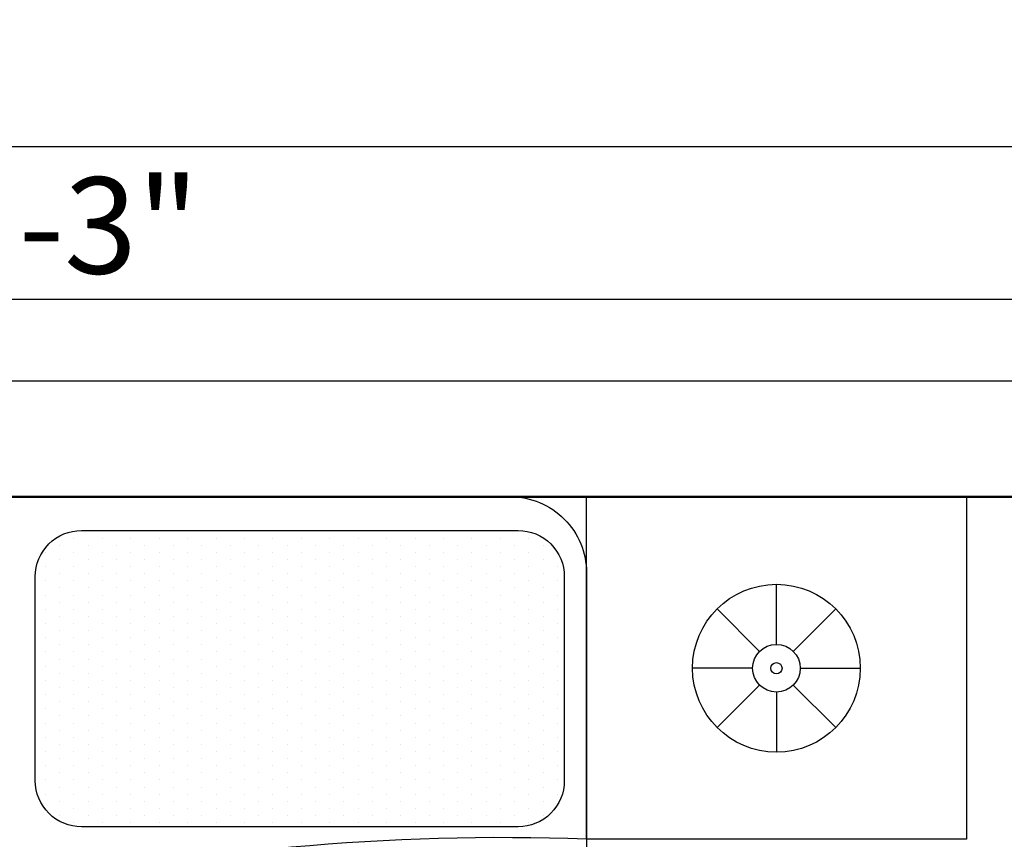
# Model space of a CAD drawing. Units: inches. Extents: x 3064 to 19385, y 846 to 15425.
# Tile 33 of 108: x 5003 to 5054, y 1368 to 1411. Entities that reach past the tile are written whole.
import ezdxf

# ---------------------------------------------------------------- set-up
doc = ezdxf.new("R2010")
doc.units = ezdxf.units.IN
for name, color, linetype, lineweight in [('A-ANNO-DIMS', 2, 'Continuous', 18), ('A-FLOR-FIXT', 9, 'Continuous', 18), ('A-WALL', 7, 'Continuous', 50), ('C-PROP', 6, 'Continuous', 25)]:
    doc.layers.add(name, color=color, linetype=linetype, lineweight=lineweight)
doc.layers.add('BLOCK', color=6, linetype='Continuous')
doc.styles.get("Standard").update_dxf_attribs({"font": 'arial.ttf'})
doc.dimstyles.new('ISO-25', dxfattribs={"dimtxt": 9, "dimasz": 2.5, "dimexe": 1.25, "dimexo": 0.625, "dimtad": 1, "dimdec": 1, "dimlunit": 3, "dimtxsty": 'Standard', "dimcen": 2.5, "dimadec": 0, "dimazin": 0, "dimtfac": 1, "dimtdec": 1, "dimtmove": 0, "dimatfit": 3, "dimfxl": 1, "dimarcsym": 0})

# ---------------------------------------------------------------- blocks, each defined once
blk = doc.blocks.new('*X7')
at = {"color": 0}
for p, q in [((273.75, 456.9375), (273.75, 456.9375)), ((273.9375, 457.03125), (273.9375, 457.03125)), ((274.125, 456.9375), (274.125, 456.9375)), ((274.3125, 457.03125), (274.3125, 457.03125)), ((274.5, 456.9375), (274.5, 456.9375)), ((274.6875, 457.03125), (274.6875, 457.03125)), ((274.875, 456.9375), (274.875, 456.9375)), ((275.0625, 457.03125), (275.0625, 457.03125)), ((275.25, 456.9375), (275.25, 456.9375)), ((275.4375, 457.03125), (275.4375, 457.03125)), ((275.625, 456.9375), (275.625, 456.9375)), ((275.8125, 457.03125), (275.8125, 457.03125)), ((276, 456.9375), (276, 456.9375)), ((276.1875, 457.03125), (276.1875, 457.03125)), ((276.375, 456.9375), (276.375, 456.9375)), ((276.5625, 457.03125), (276.5625, 457.03125)), ((276.75, 456.9375), (276.75, 456.9375)), ((276.9375, 457.03125), (276.9375, 457.03125)), ((277.125, 456.9375), (277.125, 456.9375)), ((277.3125, 457.03125), (277.3125, 457.03125)), ((277.5, 456.9375), (277.5, 456.9375)), ((277.6875, 457.03125), (277.6875, 457.03125)), ((277.875, 456.9375), (277.875, 456.9375)), ((278.0625, 457.03125), (278.0625, 457.03125)), ((278.25, 456.9375), (278.25, 456.9375)), ((278.4375, 457.03125), (278.4375, 457.03125)), ((278.625, 456.9375), (278.625, 456.9375)), ((278.8125, 457.03125), (278.8125, 457.03125)), ((279, 456.9375), (279, 456.9375)), ((279.1875, 457.03125), (279.1875, 457.03125)), ((279.375, 456.9375), (279.375, 456.9375)), ((279.5625, 457.03125), (279.5625, 457.03125)), ((279.75, 456.9375), (279.75, 456.9375)), ((273.5625, 456.84375), (273.5625, 456.84375)), ((273.9375, 456.84375), (273.9375, 456.84375)), ((274.3125, 456.84375), (274.3125, 456.84375)), ((274.6875, 456.84375), (274.6875, 456.84375)), ((275.0625, 456.84375), (275.0625, 456.84375)), ((275.4375, 456.84375), (275.4375, 456.84375)), ((275.8125, 456.84375), (275.8125, 456.84375)), ((276.1875, 456.84375), (276.1875, 456.84375)), ((276.5625, 456.84375), (276.5625, 456.84375)), ((276.9375, 456.84375), (276.9375, 456.84375)), ((277.3125, 456.84375), (277.3125, 456.84375)), ((277.6875, 456.84375), (277.6875, 456.84375)), ((278.0625, 456.84375), (278.0625, 456.84375)), ((278.4375, 456.84375), (278.4375, 456.84375)), ((278.8125, 456.84375), (278.8125, 456.84375)), ((279.1875, 456.84375), (279.1875, 456.84375)), ((279.5625, 456.84375), (279.5625, 456.84375)), ((279.9375, 456.84375), (279.9375, 456.84375)), ((273.375, 456.75), (273.375, 456.75)), ((273.5625, 456.65625), (273.5625, 456.65625)), ((273.75, 456.75), (273.75, 456.75)), ((273.9375, 456.65625), (273.9375, 456.65625)), ((274.125, 456.75), (274.125, 456.75)), ((274.3125, 456.65625), (274.3125, 456.65625)), ((274.5, 456.75), (274.5, 456.75)), ((274.6875, 456.65625), (274.6875, 456.65625)), ((274.875, 456.75), (274.875, 456.75)), ((275.0625, 456.65625), (275.0625, 456.65625)), ((275.25, 456.75), (275.25, 456.75)), ((275.4375, 456.65625), (275.4375, 456.65625)), ((275.625, 456.75), (275.625, 456.75)), ((275.8125, 456.65625), (275.8125, 456.65625)), ((276, 456.75), (276, 456.75)), ((276.1875, 456.65625), (276.1875, 456.65625)), ((276.375, 456.75), (276.375, 456.75)), ((276.5625, 456.65625), (276.5625, 456.65625)), ((276.75, 456.75), (276.75, 456.75)), ((276.9375, 456.65625), (276.9375, 456.65625)), ((277.125, 456.75), (277.125, 456.75)), ((277.3125, 456.65625), (277.3125, 456.65625)), ((277.5, 456.75), (277.5, 456.75)), ((277.6875, 456.65625), (277.6875, 456.65625)), ((277.875, 456.75), (277.875, 456.75)), ((278.0625, 456.65625), (278.0625, 456.65625)), ((278.25, 456.75), (278.25, 456.75)), ((278.4375, 456.65625), (278.4375, 456.65625)), ((278.625, 456.75), (278.625, 456.75)), ((278.8125, 456.65625), (278.8125, 456.65625)), ((279, 456.75), (279, 456.75)), ((279.1875, 456.65625), (279.1875, 456.65625)), ((279.375, 456.75), (279.375, 456.75)), ((279.5625, 456.65625), (279.5625, 456.65625)), ((279.75, 456.75), (279.75, 456.75)), ((279.9375, 456.65625), (279.9375, 456.65625)), ((280.125, 456.75), (280.125, 456.75)), ((273.375, 456.5625), (273.375, 456.5625)), ((273.75, 456.5625), (273.75, 456.5625)), ((274.125, 456.5625), (274.125, 456.5625)), ((274.5, 456.5625), (274.5, 456.5625)), ((274.875, 456.5625), (274.875, 456.5625)), ((275.25, 456.5625), (275.25, 456.5625)), ((275.625, 456.5625), (275.625, 456.5625)), ((276, 456.5625), (276, 456.5625)), ((276.375, 456.5625), (276.375, 456.5625)), ((276.75, 456.5625), (276.75, 456.5625)), ((277.125, 456.5625), (277.125, 456.5625)), ((277.5, 456.5625), (277.5, 456.5625)), ((277.875, 456.5625), (277.875, 456.5625)), ((278.25, 456.5625), (278.25, 456.5625)), ((278.625, 456.5625), (278.625, 456.5625)), ((279, 456.5625), (279, 456.5625)), ((279.375, 456.5625), (279.375, 456.5625)), ((279.75, 456.5625), (279.75, 456.5625)), ((280.125, 456.5625), (280.125, 456.5625)), ((273.5625, 456.46875), (273.5625, 456.46875)), ((273.9375, 456.46875), (273.9375, 456.46875)), ((274.3125, 456.46875), (274.3125, 456.46875)), ((274.6875, 456.46875), (274.6875, 456.46875)), ((275.0625, 456.46875), (275.0625, 456.46875)), ((275.4375, 456.46875), (275.4375, 456.46875)), ((275.8125, 456.46875), (275.8125, 456.46875)), ((276.1875, 456.46875), (276.1875, 456.46875)), ((276.5625, 456.46875), (276.5625, 456.46875)), ((276.9375, 456.46875), (276.9375, 456.46875)), ((277.3125, 456.46875), (277.3125, 456.46875)), ((277.6875, 456.46875), (277.6875, 456.46875)), ((278.0625, 456.46875), (278.0625, 456.46875)), ((278.4375, 456.46875), (278.4375, 456.46875)), ((278.8125, 456.46875), (278.8125, 456.46875)), ((279.1875, 456.46875), (279.1875, 456.46875)), ((279.5625, 456.46875), (279.5625, 456.46875)), ((279.9375, 456.46875), (279.9375, 456.46875)), ((273.375, 456.375), (273.375, 456.375)), ((273.5625, 456.28125), (273.5625, 456.28125)), ((273.75, 456.375), (273.75, 456.375)), ((273.9375, 456.28125), (273.9375, 456.28125)), ((274.125, 456.375), (274.125, 456.375)), ((274.3125, 456.28125), (274.3125, 456.28125)), ((274.5, 456.375), (274.5, 456.375)), ((274.6875, 456.28125), (274.6875, 456.28125)), ((274.875, 456.375), (274.875, 456.375)), ((275.0625, 456.28125), (275.0625, 456.28125)), ((275.25, 456.375), (275.25, 456.375)), ((275.4375, 456.28125), (275.4375, 456.28125)), ((275.625, 456.375), (275.625, 456.375)), ((275.8125, 456.28125), (275.8125, 456.28125)), ((276, 456.375), (276, 456.375)), ((276.1875, 456.28125), (276.1875, 456.28125)), ((276.375, 456.375), (276.375, 456.375)), ((276.5625, 456.28125), (276.5625, 456.28125)), ((276.75, 456.375), (276.75, 456.375)), ((276.9375, 456.28125), (276.9375, 456.28125)), ((277.125, 456.375), (277.125, 456.375)), ((277.3125, 456.28125), (277.3125, 456.28125)), ((277.5, 456.375), (277.5, 456.375)), ((277.6875, 456.28125), (277.6875, 456.28125)), ((277.875, 456.375), (277.875, 456.375)), ((278.0625, 456.28125), (278.0625, 456.28125)), ((278.25, 456.375), (278.25, 456.375)), ((278.4375, 456.28125), (278.4375, 456.28125)), ((278.625, 456.375), (278.625, 456.375)), ((278.8125, 456.28125), (278.8125, 456.28125)), ((279, 456.375), (279, 456.375)), ((279.1875, 456.28125), (279.1875, 456.28125)), ((279.375, 456.375), (279.375, 456.375)), ((279.5625, 456.28125), (279.5625, 456.28125)), ((279.75, 456.375), (279.75, 456.375)), ((279.9375, 456.28125), (279.9375, 456.28125)), ((280.125, 456.375), (280.125, 456.375)), ((273.375, 456.1875), (273.375, 456.1875)), ((273.75, 456.1875), (273.75, 456.1875)), ((274.125, 456.1875), (274.125, 456.1875)), ((274.5, 456.1875), (274.5, 456.1875)), ((274.875, 456.1875), (274.875, 456.1875)), ((275.25, 456.1875), (275.25, 456.1875)), ((275.625, 456.1875), (275.625, 456.1875)), ((276, 456.1875), (276, 456.1875)), ((276.375, 456.1875), (276.375, 456.1875)), ((276.75, 456.1875), (276.75, 456.1875)), ((277.125, 456.1875), (277.125, 456.1875)), ((277.5, 456.1875), (277.5, 456.1875)), ((277.875, 456.1875), (277.875, 456.1875)), ((278.25, 456.1875), (278.25, 456.1875)), ((278.625, 456.1875), (278.625, 456.1875)), ((279, 456.1875), (279, 456.1875)), ((279.375, 456.1875), (279.375, 456.1875)), ((279.75, 456.1875), (279.75, 456.1875)), ((280.125, 456.1875), (280.125, 456.1875)), ((273.375, 456), (273.375, 456)), ((273.5625, 456.09375), (273.5625, 456.09375)), ((273.75, 456), (273.75, 456)), ((273.9375, 456.09375), (273.9375, 456.09375)), ((274.125, 456), (274.125, 456)), ((274.3125, 456.09375), (274.3125, 456.09375)), ((274.5, 456), (274.5, 456)), ((274.6875, 456.09375), (274.6875, 456.09375)), ((274.875, 456), (274.875, 456)), ((275.0625, 456.09375), (275.0625, 456.09375)), ((275.25, 456), (275.25, 456)), ((275.4375, 456.09375), (275.4375, 456.09375)), ((275.625, 456), (275.625, 456)), ((275.8125, 456.09375), (275.8125, 456.09375)), ((276, 456), (276, 456)), ((276.1875, 456.09375), (276.1875, 456.09375)), ((276.375, 456), (276.375, 456)), ((276.5625, 456.09375), (276.5625, 456.09375)), ((276.75, 456), (276.75, 456)), ((276.9375, 456.09375), (276.9375, 456.09375)), ((277.125, 456), (277.125, 456)), ((277.3125, 456.09375), (277.3125, 456.09375)), ((277.5, 456), (277.5, 456)), ((277.6875, 456.09375), (277.6875, 456.09375)), ((277.875, 456), (277.875, 456)), ((278.0625, 456.09375), (278.0625, 456.09375)), ((278.25, 456), (278.25, 456)), ((278.4375, 456.09375), (278.4375, 456.09375)), ((278.625, 456), (278.625, 456)), ((278.8125, 456.09375), (278.8125, 456.09375)), ((279, 456), (279, 456)), ((279.1875, 456.09375), (279.1875, 456.09375)), ((279.375, 456), (279.375, 456)), ((279.5625, 456.09375), (279.5625, 456.09375)), ((279.75, 456), (279.75, 456)), ((279.9375, 456.09375), (279.9375, 456.09375)), ((280.125, 456), (280.125, 456)), ((273.5625, 455.90625), (273.5625, 455.90625)), ((273.9375, 455.90625), (273.9375, 455.90625)), ((274.3125, 455.90625), (274.3125, 455.90625)), ((274.6875, 455.90625), (274.6875, 455.90625)), ((275.0625, 455.90625), (275.0625, 455.90625)), ((275.4375, 455.90625), (275.4375, 455.90625)), ((275.8125, 455.90625), (275.8125, 455.90625)), ((276.1875, 455.90625), (276.1875, 455.90625)), ((276.5625, 455.90625), (276.5625, 455.90625)), ((276.9375, 455.90625), (276.9375, 455.90625)), ((277.3125, 455.90625), (277.3125, 455.90625)), ((277.6875, 455.90625), (277.6875, 455.90625)), ((278.0625, 455.90625), (278.0625, 455.90625)), ((278.4375, 455.90625), (278.4375, 455.90625)), ((278.8125, 455.90625), (278.8125, 455.90625)), ((279.1875, 455.90625), (279.1875, 455.90625)), ((279.5625, 455.90625), (279.5625, 455.90625)), ((279.9375, 455.90625), (279.9375, 455.90625)), ((273.375, 455.8125), (273.375, 455.8125)), ((273.75, 455.8125), (273.75, 455.8125)), ((274.125, 455.8125), (274.125, 455.8125)), ((274.5, 455.8125), (274.5, 455.8125)), ((274.875, 455.8125), (274.875, 455.8125)), ((275.25, 455.8125), (275.25, 455.8125)), ((275.625, 455.8125), (275.625, 455.8125)), ((276, 455.8125), (276, 455.8125)), ((276.375, 455.8125), (276.375, 455.8125)), ((276.75, 455.8125), (276.75, 455.8125)), ((277.125, 455.8125), (277.125, 455.8125)), ((277.5, 455.8125), (277.5, 455.8125)), ((277.875, 455.8125), (277.875, 455.8125)), ((278.25, 455.8125), (278.25, 455.8125)), ((278.625, 455.8125), (278.625, 455.8125)), ((279, 455.8125), (279, 455.8125)), ((279.375, 455.8125), (279.375, 455.8125)), ((279.75, 455.8125), (279.75, 455.8125)), ((280.125, 455.8125), (280.125, 455.8125)), ((273.375, 455.625), (273.375, 455.625)), ((273.5625, 455.71875), (273.5625, 455.71875)), ((273.75, 455.625), (273.75, 455.625)), ((273.9375, 455.71875), (273.9375, 455.71875)), ((274.125, 455.625), (274.125, 455.625)), ((274.3125, 455.71875), (274.3125, 455.71875)), ((274.5, 455.625), (274.5, 455.625)), ((274.6875, 455.71875), (274.6875, 455.71875)), ((274.875, 455.625), (274.875, 455.625)), ((275.0625, 455.71875), (275.0625, 455.71875)), ((275.25, 455.625), (275.25, 455.625)), ((275.4375, 455.71875), (275.4375, 455.71875)), ((275.625, 455.625), (275.625, 455.625)), ((275.8125, 455.71875), (275.8125, 455.71875)), ((276, 455.625), (276, 455.625)), ((276.1875, 455.71875), (276.1875, 455.71875)), ((276.375, 455.625), (276.375, 455.625)), ((276.5625, 455.71875), (276.5625, 455.71875)), ((276.75, 455.625), (276.75, 455.625)), ((276.9375, 455.71875), (276.9375, 455.71875)), ((277.125, 455.625), (277.125, 455.625)), ((277.3125, 455.71875), (277.3125, 455.71875)), ((277.5, 455.625), (277.5, 455.625)), ((277.6875, 455.71875), (277.6875, 455.71875)), ((277.875, 455.625), (277.875, 455.625)), ((278.0625, 455.71875), (278.0625, 455.71875)), ((278.25, 455.625), (278.25, 455.625)), ((278.4375, 455.71875), (278.4375, 455.71875)), ((278.625, 455.625), (278.625, 455.625)), ((278.8125, 455.71875), (278.8125, 455.71875)), ((279, 455.625), (279, 455.625)), ((279.1875, 455.71875), (279.1875, 455.71875)), ((279.375, 455.625), (279.375, 455.625)), ((279.5625, 455.71875), (279.5625, 455.71875)), ((279.75, 455.625), (279.75, 455.625)), ((279.9375, 455.71875), (279.9375, 455.71875)), ((280.125, 455.625), (280.125, 455.625)), ((273.5625, 455.53125), (273.5625, 455.53125)), ((273.9375, 455.53125), (273.9375, 455.53125)), ((274.3125, 455.53125), (274.3125, 455.53125)), ((274.6875, 455.53125), (274.6875, 455.53125)), ((275.0625, 455.53125), (275.0625, 455.53125)), ((275.4375, 455.53125), (275.4375, 455.53125)), ((275.8125, 455.53125), (275.8125, 455.53125)), ((276.1875, 455.53125), (276.1875, 455.53125)), ((276.5625, 455.53125), (276.5625, 455.53125)), ((276.9375, 455.53125), (276.9375, 455.53125)), ((277.3125, 455.53125), (277.3125, 455.53125)), ((277.6875, 455.53125), (277.6875, 455.53125)), ((278.0625, 455.53125), (278.0625, 455.53125)), ((278.4375, 455.53125), (278.4375, 455.53125)), ((278.8125, 455.53125), (278.8125, 455.53125)), ((279.1875, 455.53125), (279.1875, 455.53125)), ((279.5625, 455.53125), (279.5625, 455.53125)), ((279.9375, 455.53125), (279.9375, 455.53125)), ((273.375, 455.4375), (273.375, 455.4375)), ((273.75, 455.4375), (273.75, 455.4375)), ((274.125, 455.4375), (274.125, 455.4375)), ((274.5, 455.4375), (274.5, 455.4375)), ((274.875, 455.4375), (274.875, 455.4375)), ((275.25, 455.4375), (275.25, 455.4375)), ((275.625, 455.4375), (275.625, 455.4375)), ((276, 455.4375), (276, 455.4375)), ((276.375, 455.4375), (276.375, 455.4375)), ((276.75, 455.4375), (276.75, 455.4375)), ((277.125, 455.4375), (277.125, 455.4375)), ((277.5, 455.4375), (277.5, 455.4375)), ((277.875, 455.4375), (277.875, 455.4375)), ((278.25, 455.4375), (278.25, 455.4375)), ((278.625, 455.4375), (278.625, 455.4375)), ((279, 455.4375), (279, 455.4375)), ((279.375, 455.4375), (279.375, 455.4375)), ((279.75, 455.4375), (279.75, 455.4375)), ((280.125, 455.4375), (280.125, 455.4375)), ((273.375, 455.25), (273.375, 455.25)), ((273.5625, 455.34375), (273.5625, 455.34375)), ((273.75, 455.25), (273.75, 455.25)), ((273.9375, 455.34375), (273.9375, 455.34375)), ((274.125, 455.25), (274.125, 455.25)), ((274.3125, 455.34375), (274.3125, 455.34375)), ((274.5, 455.25), (274.5, 455.25)), ((274.6875, 455.34375), (274.6875, 455.34375)), ((274.875, 455.25), (274.875, 455.25)), ((275.0625, 455.34375), (275.0625, 455.34375)), ((275.25, 455.25), (275.25, 455.25)), ((275.4375, 455.34375), (275.4375, 455.34375)), ((275.625, 455.25), (275.625, 455.25)), ((275.8125, 455.34375), (275.8125, 455.34375)), ((276, 455.25), (276, 455.25)), ((276.1875, 455.34375), (276.1875, 455.34375)), ((276.375, 455.25), (276.375, 455.25)), ((276.5625, 455.34375), (276.5625, 455.34375)), ((276.75, 455.25), (276.75, 455.25)), ((276.9375, 455.34375), (276.9375, 455.34375)), ((277.125, 455.25), (277.125, 455.25)), ((277.3125, 455.34375), (277.3125, 455.34375)), ((277.5, 455.25), (277.5, 455.25)), ((277.6875, 455.34375), (277.6875, 455.34375)), ((277.875, 455.25), (277.875, 455.25)), ((278.0625, 455.34375), (278.0625, 455.34375)), ((278.25, 455.25), (278.25, 455.25)), ((278.4375, 455.34375), (278.4375, 455.34375)), ((278.625, 455.25), (278.625, 455.25)), ((278.8125, 455.34375), (278.8125, 455.34375)), ((279, 455.25), (279, 455.25)), ((279.1875, 455.34375), (279.1875, 455.34375)), ((279.375, 455.25), (279.375, 455.25)), ((279.5625, 455.34375), (279.5625, 455.34375)), ((279.75, 455.25), (279.75, 455.25)), ((279.9375, 455.34375), (279.9375, 455.34375)), ((280.125, 455.25), (280.125, 455.25)), ((273.5625, 455.15625), (273.5625, 455.15625)), ((273.9375, 455.15625), (273.9375, 455.15625)), ((274.3125, 455.15625), (274.3125, 455.15625)), ((274.6875, 455.15625), (274.6875, 455.15625)), ((275.0625, 455.15625), (275.0625, 455.15625)), ((275.4375, 455.15625), (275.4375, 455.15625)), ((275.8125, 455.15625), (275.8125, 455.15625)), ((276.1875, 455.15625), (276.1875, 455.15625)), ((276.5625, 455.15625), (276.5625, 455.15625)), ((276.9375, 455.15625), (276.9375, 455.15625)), ((277.3125, 455.15625), (277.3125, 455.15625)), ((277.6875, 455.15625), (277.6875, 455.15625)), ((278.0625, 455.15625), (278.0625, 455.15625)), ((278.4375, 455.15625), (278.4375, 455.15625)), ((278.8125, 455.15625), (278.8125, 455.15625)), ((279.1875, 455.15625), (279.1875, 455.15625)), ((279.5625, 455.15625), (279.5625, 455.15625)), ((279.9375, 455.15625), (279.9375, 455.15625)), ((273.375, 455.0625), (273.375, 455.0625)), ((273.5625, 454.96875), (273.5625, 454.96875)), ((273.75, 455.0625), (273.75, 455.0625)), ((273.9375, 454.96875), (273.9375, 454.96875)), ((274.125, 455.0625), (274.125, 455.0625)), ((274.3125, 454.96875), (274.3125, 454.96875)), ((274.5, 455.0625), (274.5, 455.0625)), ((274.6875, 454.96875), (274.6875, 454.96875)), ((274.875, 455.0625), (274.875, 455.0625)), ((275.0625, 454.96875), (275.0625, 454.96875)), ((275.25, 455.0625), (275.25, 455.0625)), ((275.4375, 454.96875), (275.4375, 454.96875)), ((275.625, 455.0625), (275.625, 455.0625)), ((275.8125, 454.96875), (275.8125, 454.96875)), ((276, 455.0625), (276, 455.0625)), ((276.1875, 454.96875), (276.1875, 454.96875)), ((276.375, 455.0625), (276.375, 455.0625)), ((276.5625, 454.96875), (276.5625, 454.96875)), ((276.75, 455.0625), (276.75, 455.0625)), ((276.9375, 454.96875), (276.9375, 454.96875)), ((277.125, 455.0625), (277.125, 455.0625)), ((277.3125, 454.96875), (277.3125, 454.96875)), ((277.5, 455.0625), (277.5, 455.0625)), ((277.6875, 454.96875), (277.6875, 454.96875)), ((277.875, 455.0625), (277.875, 455.0625)), ((278.0625, 454.96875), (278.0625, 454.96875)), ((278.25, 455.0625), (278.25, 455.0625)), ((278.4375, 454.96875), (278.4375, 454.96875)), ((278.625, 455.0625), (278.625, 455.0625)), ((278.8125, 454.96875), (278.8125, 454.96875)), ((279, 455.0625), (279, 455.0625)), ((279.1875, 454.96875), (279.1875, 454.96875)), ((279.375, 455.0625), (279.375, 455.0625)), ((279.5625, 454.96875), (279.5625, 454.96875)), ((279.75, 455.0625), (279.75, 455.0625)), ((279.9375, 454.96875), (279.9375, 454.96875)), ((280.125, 455.0625), (280.125, 455.0625)), ((273.375, 454.875), (273.375, 454.875)), ((273.75, 454.875), (273.75, 454.875)), ((274.125, 454.875), (274.125, 454.875)), ((274.5, 454.875), (274.5, 454.875)), ((274.875, 454.875), (274.875, 454.875)), ((275.25, 454.875), (275.25, 454.875)), ((275.625, 454.875), (275.625, 454.875)), ((276, 454.875), (276, 454.875)), ((276.375, 454.875), (276.375, 454.875)), ((276.75, 454.875), (276.75, 454.875)), ((277.125, 454.875), (277.125, 454.875)), ((277.5, 454.875), (277.5, 454.875)), ((277.875, 454.875), (277.875, 454.875)), ((278.25, 454.875), (278.25, 454.875)), ((278.625, 454.875), (278.625, 454.875)), ((279, 454.875), (279, 454.875)), ((279.375, 454.875), (279.375, 454.875)), ((279.75, 454.875), (279.75, 454.875)), ((280.125, 454.875), (280.125, 454.875)), ((273.5625, 454.78125), (273.5625, 454.78125)), ((273.9375, 454.78125), (273.9375, 454.78125)), ((274.3125, 454.78125), (274.3125, 454.78125)), ((274.6875, 454.78125), (274.6875, 454.78125)), ((275.0625, 454.78125), (275.0625, 454.78125)), ((275.4375, 454.78125), (275.4375, 454.78125)), ((275.8125, 454.78125), (275.8125, 454.78125)), ((276.1875, 454.78125), (276.1875, 454.78125)), ((276.5625, 454.78125), (276.5625, 454.78125)), ((276.9375, 454.78125), (276.9375, 454.78125)), ((277.3125, 454.78125), (277.3125, 454.78125)), ((277.6875, 454.78125), (277.6875, 454.78125)), ((278.0625, 454.78125), (278.0625, 454.78125)), ((278.4375, 454.78125), (278.4375, 454.78125)), ((278.8125, 454.78125), (278.8125, 454.78125)), ((279.1875, 454.78125), (279.1875, 454.78125)), ((279.5625, 454.78125), (279.5625, 454.78125)), ((279.9375, 454.78125), (279.9375, 454.78125)), ((273.375, 454.6875), (273.375, 454.6875)), ((273.5625, 454.59375), (273.5625, 454.59375)), ((273.75, 454.6875), (273.75, 454.6875)), ((273.9375, 454.59375), (273.9375, 454.59375)), ((274.125, 454.6875), (274.125, 454.6875)), ((274.3125, 454.59375), (274.3125, 454.59375)), ((274.5, 454.6875), (274.5, 454.6875)), ((274.6875, 454.59375), (274.6875, 454.59375)), ((274.875, 454.6875), (274.875, 454.6875)), ((275.0625, 454.59375), (275.0625, 454.59375)), ((275.25, 454.6875), (275.25, 454.6875)), ((275.4375, 454.59375), (275.4375, 454.59375)), ((275.625, 454.6875), (275.625, 454.6875)), ((275.8125, 454.59375), (275.8125, 454.59375)), ((276, 454.6875), (276, 454.6875)), ((276.1875, 454.59375), (276.1875, 454.59375)), ((276.375, 454.6875), (276.375, 454.6875)), ((276.5625, 454.59375), (276.5625, 454.59375)), ((276.75, 454.6875), (276.75, 454.6875)), ((276.9375, 454.59375), (276.9375, 454.59375)), ((277.125, 454.6875), (277.125, 454.6875)), ((277.3125, 454.59375), (277.3125, 454.59375)), ((277.5, 454.6875), (277.5, 454.6875)), ((277.6875, 454.59375), (277.6875, 454.59375)), ((277.875, 454.6875), (277.875, 454.6875)), ((278.0625, 454.59375), (278.0625, 454.59375)), ((278.25, 454.6875), (278.25, 454.6875)), ((278.4375, 454.59375), (278.4375, 454.59375)), ((278.625, 454.6875), (278.625, 454.6875)), ((278.8125, 454.59375), (278.8125, 454.59375)), ((279, 454.6875), (279, 454.6875)), ((279.1875, 454.59375), (279.1875, 454.59375)), ((279.375, 454.6875), (279.375, 454.6875)), ((279.5625, 454.59375), (279.5625, 454.59375)), ((279.75, 454.6875), (279.75, 454.6875)), ((279.9375, 454.59375), (279.9375, 454.59375)), ((280.125, 454.6875), (280.125, 454.6875)), ((273.375, 454.5), (273.375, 454.5)), ((273.75, 454.5), (273.75, 454.5)), ((274.125, 454.5), (274.125, 454.5)), ((274.5, 454.5), (274.5, 454.5)), ((274.875, 454.5), (274.875, 454.5)), ((275.25, 454.5), (275.25, 454.5)), ((275.625, 454.5), (275.625, 454.5)), ((276, 454.5), (276, 454.5)), ((276.375, 454.5), (276.375, 454.5)), ((276.75, 454.5), (276.75, 454.5)), ((277.125, 454.5), (277.125, 454.5)), ((277.5, 454.5), (277.5, 454.5)), ((277.875, 454.5), (277.875, 454.5)), ((278.25, 454.5), (278.25, 454.5)), ((278.625, 454.5), (278.625, 454.5)), ((279, 454.5), (279, 454.5)), ((279.375, 454.5), (279.375, 454.5)), ((279.75, 454.5), (279.75, 454.5)), ((280.125, 454.5), (280.125, 454.5)), ((273.375, 454.3125), (273.375, 454.3125)), ((273.5625, 454.40625), (273.5625, 454.40625)), ((273.75, 454.3125), (273.75, 454.3125)), ((273.9375, 454.40625), (273.9375, 454.40625)), ((274.125, 454.3125), (274.125, 454.3125)), ((274.3125, 454.40625), (274.3125, 454.40625)), ((274.5, 454.3125), (274.5, 454.3125)), ((274.6875, 454.40625), (274.6875, 454.40625)), ((274.875, 454.3125), (274.875, 454.3125)), ((275.0625, 454.40625), (275.0625, 454.40625)), ((275.25, 454.3125), (275.25, 454.3125)), ((275.4375, 454.40625), (275.4375, 454.40625)), ((275.625, 454.3125), (275.625, 454.3125)), ((275.8125, 454.40625), (275.8125, 454.40625)), ((276, 454.3125), (276, 454.3125)), ((276.1875, 454.40625), (276.1875, 454.40625)), ((276.375, 454.3125), (276.375, 454.3125)), ((276.5625, 454.40625), (276.5625, 454.40625)), ((276.75, 454.3125), (276.75, 454.3125)), ((276.9375, 454.40625), (276.9375, 454.40625)), ((277.125, 454.3125), (277.125, 454.3125)), ((277.3125, 454.40625), (277.3125, 454.40625)), ((277.5, 454.3125), (277.5, 454.3125)), ((277.6875, 454.40625), (277.6875, 454.40625)), ((277.875, 454.3125), (277.875, 454.3125)), ((278.0625, 454.40625), (278.0625, 454.40625)), ((278.25, 454.3125), (278.25, 454.3125)), ((278.4375, 454.40625), (278.4375, 454.40625)), ((278.625, 454.3125), (278.625, 454.3125)), ((278.8125, 454.40625), (278.8125, 454.40625)), ((279, 454.3125), (279, 454.3125)), ((279.1875, 454.40625), (279.1875, 454.40625)), ((279.375, 454.3125), (279.375, 454.3125)), ((279.5625, 454.40625), (279.5625, 454.40625)), ((279.75, 454.3125), (279.75, 454.3125)), ((279.9375, 454.40625), (279.9375, 454.40625)), ((280.125, 454.3125), (280.125, 454.3125)), ((273.5625, 454.21875), (273.5625, 454.21875)), ((273.9375, 454.21875), (273.9375, 454.21875)), ((274.3125, 454.21875), (274.3125, 454.21875)), ((274.6875, 454.21875), (274.6875, 454.21875)), ((275.0625, 454.21875), (275.0625, 454.21875)), ((275.4375, 454.21875), (275.4375, 454.21875)), ((275.8125, 454.21875), (275.8125, 454.21875)), ((276.1875, 454.21875), (276.1875, 454.21875)), ((276.5625, 454.21875), (276.5625, 454.21875)), ((276.9375, 454.21875), (276.9375, 454.21875)), ((277.3125, 454.21875), (277.3125, 454.21875)), ((277.6875, 454.21875), (277.6875, 454.21875)), ((278.0625, 454.21875), (278.0625, 454.21875)), ((278.4375, 454.21875), (278.4375, 454.21875)), ((278.8125, 454.21875), (278.8125, 454.21875)), ((279.1875, 454.21875), (279.1875, 454.21875)), ((279.5625, 454.21875), (279.5625, 454.21875)), ((279.9375, 454.21875), (279.9375, 454.21875)), ((273.375, 454.125), (273.375, 454.125)), ((273.75, 454.125), (273.75, 454.125)), ((274.125, 454.125), (274.125, 454.125)), ((274.5, 454.125), (274.5, 454.125)), ((274.875, 454.125), (274.875, 454.125)), ((275.25, 454.125), (275.25, 454.125)), ((275.625, 454.125), (275.625, 454.125)), ((276, 454.125), (276, 454.125)), ((276.375, 454.125), (276.375, 454.125)), ((276.75, 454.125), (276.75, 454.125)), ((277.125, 454.125), (277.125, 454.125)), ((277.5, 454.125), (277.5, 454.125)), ((277.875, 454.125), (277.875, 454.125)), ((278.25, 454.125), (278.25, 454.125)), ((278.625, 454.125), (278.625, 454.125)), ((279, 454.125), (279, 454.125)), ((279.375, 454.125), (279.375, 454.125)), ((279.75, 454.125), (279.75, 454.125)), ((280.125, 454.125), (280.125, 454.125)), ((273.375, 453.9375), (273.375, 453.9375)), ((273.5625, 454.03125), (273.5625, 454.03125)), ((273.75, 453.9375), (273.75, 453.9375)), ((273.9375, 454.03125), (273.9375, 454.03125)), ((274.125, 453.9375), (274.125, 453.9375)), ((274.3125, 454.03125), (274.3125, 454.03125)), ((274.5, 453.9375), (274.5, 453.9375)), ((274.6875, 454.03125), (274.6875, 454.03125)), ((274.875, 453.9375), (274.875, 453.9375)), ((275.0625, 454.03125), (275.0625, 454.03125)), ((275.25, 453.9375), (275.25, 453.9375)), ((275.4375, 454.03125), (275.4375, 454.03125)), ((275.625, 453.9375), (275.625, 453.9375)), ((275.8125, 454.03125), (275.8125, 454.03125)), ((276, 453.9375), (276, 453.9375)), ((276.1875, 454.03125), (276.1875, 454.03125)), ((276.375, 453.9375), (276.375, 453.9375)), ((276.5625, 454.03125), (276.5625, 454.03125)), ((276.75, 453.9375), (276.75, 453.9375)), ((276.9375, 454.03125), (276.9375, 454.03125)), ((277.125, 453.9375), (277.125, 453.9375)), ((277.3125, 454.03125), (277.3125, 454.03125)), ((277.5, 453.9375), (277.5, 453.9375)), ((277.6875, 454.03125), (277.6875, 454.03125)), ((277.875, 453.9375), (277.875, 453.9375)), ((278.0625, 454.03125), (278.0625, 454.03125)), ((278.25, 453.9375), (278.25, 453.9375)), ((278.4375, 454.03125), (278.4375, 454.03125)), ((278.625, 453.9375), (278.625, 453.9375)), ((278.8125, 454.03125), (278.8125, 454.03125)), ((279, 453.9375), (279, 453.9375)), ((279.1875, 454.03125), (279.1875, 454.03125)), ((279.375, 453.9375), (279.375, 453.9375)), ((279.5625, 454.03125), (279.5625, 454.03125)), ((279.75, 453.9375), (279.75, 453.9375)), ((279.9375, 454.03125), (279.9375, 454.03125)), ((280.125, 453.9375), (280.125, 453.9375)), ((273.5625, 453.84375), (273.5625, 453.84375)), ((273.9375, 453.84375), (273.9375, 453.84375)), ((274.3125, 453.84375), (274.3125, 453.84375)), ((274.6875, 453.84375), (274.6875, 453.84375)), ((275.0625, 453.84375), (275.0625, 453.84375)), ((275.4375, 453.84375), (275.4375, 453.84375)), ((275.8125, 453.84375), (275.8125, 453.84375)), ((276.1875, 453.84375), (276.1875, 453.84375)), ((276.5625, 453.84375), (276.5625, 453.84375)), ((276.9375, 453.84375), (276.9375, 453.84375)), ((277.3125, 453.84375), (277.3125, 453.84375)), ((277.6875, 453.84375), (277.6875, 453.84375)), ((278.0625, 453.84375), (278.0625, 453.84375)), ((278.4375, 453.84375), (278.4375, 453.84375)), ((278.8125, 453.84375), (278.8125, 453.84375)), ((279.1875, 453.84375), (279.1875, 453.84375)), ((279.5625, 453.84375), (279.5625, 453.84375)), ((279.9375, 453.84375), (279.9375, 453.84375)), ((273.375, 453.75), (273.375, 453.75)), ((273.75, 453.75), (273.75, 453.75)), ((274.125, 453.75), (274.125, 453.75)), ((274.5, 453.75), (274.5, 453.75)), ((274.875, 453.75), (274.875, 453.75)), ((275.25, 453.75), (275.25, 453.75)), ((275.625, 453.75), (275.625, 453.75)), ((276, 453.75), (276, 453.75)), ((276.375, 453.75), (276.375, 453.75)), ((276.75, 453.75), (276.75, 453.75)), ((277.125, 453.75), (277.125, 453.75)), ((277.5, 453.75), (277.5, 453.75)), ((277.875, 453.75), (277.875, 453.75)), ((278.25, 453.75), (278.25, 453.75)), ((278.625, 453.75), (278.625, 453.75)), ((279, 453.75), (279, 453.75)), ((279.375, 453.75), (279.375, 453.75)), ((279.75, 453.75), (279.75, 453.75)), ((280.125, 453.75), (280.125, 453.75)), ((273.375, 453.5625), (273.375, 453.5625)), ((273.5625, 453.65625), (273.5625, 453.65625)), ((273.75, 453.5625), (273.75, 453.5625)), ((273.9375, 453.65625), (273.9375, 453.65625)), ((274.125, 453.5625), (274.125, 453.5625)), ((274.3125, 453.65625), (274.3125, 453.65625)), ((274.5, 453.5625), (274.5, 453.5625)), ((274.6875, 453.65625), (274.6875, 453.65625)), ((274.875, 453.5625), (274.875, 453.5625)), ((275.0625, 453.65625), (275.0625, 453.65625)), ((275.25, 453.5625), (275.25, 453.5625)), ((275.4375, 453.65625), (275.4375, 453.65625)), ((275.625, 453.5625), (275.625, 453.5625)), ((275.8125, 453.65625), (275.8125, 453.65625)), ((276, 453.5625), (276, 453.5625)), ((276.1875, 453.65625), (276.1875, 453.65625)), ((276.375, 453.5625), (276.375, 453.5625)), ((276.5625, 453.65625), (276.5625, 453.65625)), ((276.75, 453.5625), (276.75, 453.5625)), ((276.9375, 453.65625), (276.9375, 453.65625)), ((277.125, 453.5625), (277.125, 453.5625)), ((277.3125, 453.65625), (277.3125, 453.65625)), ((277.5, 453.5625), (277.5, 453.5625)), ((277.6875, 453.65625), (277.6875, 453.65625)), ((277.875, 453.5625), (277.875, 453.5625)), ((278.0625, 453.65625), (278.0625, 453.65625)), ((278.25, 453.5625), (278.25, 453.5625)), ((278.4375, 453.65625), (278.4375, 453.65625)), ((278.625, 453.5625), (278.625, 453.5625)), ((278.8125, 453.65625), (278.8125, 453.65625)), ((279, 453.5625), (279, 453.5625)), ((279.1875, 453.65625), (279.1875, 453.65625)), ((279.375, 453.5625), (279.375, 453.5625)), ((279.5625, 453.65625), (279.5625, 453.65625)), ((279.75, 453.5625), (279.75, 453.5625)), ((279.9375, 453.65625), (279.9375, 453.65625)), ((280.125, 453.5625), (280.125, 453.5625)), ((273.5625, 453.46875), (273.5625, 453.46875)), ((273.9375, 453.46875), (273.9375, 453.46875)), ((274.3125, 453.46875), (274.3125, 453.46875)), ((274.6875, 453.46875), (274.6875, 453.46875)), ((275.0625, 453.46875), (275.0625, 453.46875)), ((275.4375, 453.46875), (275.4375, 453.46875)), ((275.8125, 453.46875), (275.8125, 453.46875)), ((276.1875, 453.46875), (276.1875, 453.46875)), ((276.5625, 453.46875), (276.5625, 453.46875)), ((276.9375, 453.46875), (276.9375, 453.46875)), ((277.3125, 453.46875), (277.3125, 453.46875)), ((277.6875, 453.46875), (277.6875, 453.46875)), ((278.0625, 453.46875), (278.0625, 453.46875)), ((278.4375, 453.46875), (278.4375, 453.46875)), ((278.8125, 453.46875), (278.8125, 453.46875)), ((279.1875, 453.46875), (279.1875, 453.46875)), ((279.5625, 453.46875), (279.5625, 453.46875)), ((279.9375, 453.46875), (279.9375, 453.46875)), ((273.375, 453.375), (273.375, 453.375)), ((273.5625, 453.28125), (273.5625, 453.28125)), ((273.75, 453.375), (273.75, 453.375)), ((273.9375, 453.28125), (273.9375, 453.28125)), ((274.125, 453.375), (274.125, 453.375)), ((274.3125, 453.28125), (274.3125, 453.28125)), ((274.5, 453.375), (274.5, 453.375)), ((274.6875, 453.28125), (274.6875, 453.28125)), ((274.875, 453.375), (274.875, 453.375)), ((275.0625, 453.28125), (275.0625, 453.28125)), ((275.25, 453.375), (275.25, 453.375)), ((275.4375, 453.28125), (275.4375, 453.28125)), ((275.625, 453.375), (275.625, 453.375)), ((275.8125, 453.28125), (275.8125, 453.28125)), ((276, 453.375), (276, 453.375)), ((276.1875, 453.28125), (276.1875, 453.28125)), ((276.375, 453.375), (276.375, 453.375)), ((276.5625, 453.28125), (276.5625, 453.28125)), ((276.75, 453.375), (276.75, 453.375)), ((276.9375, 453.28125), (276.9375, 453.28125)), ((277.125, 453.375), (277.125, 453.375)), ((277.3125, 453.28125), (277.3125, 453.28125)), ((277.5, 453.375), (277.5, 453.375)), ((277.6875, 453.28125), (277.6875, 453.28125)), ((277.875, 453.375), (277.875, 453.375)), ((278.0625, 453.28125), (278.0625, 453.28125)), ((278.25, 453.375), (278.25, 453.375)), ((278.4375, 453.28125), (278.4375, 453.28125)), ((278.625, 453.375), (278.625, 453.375)), ((278.8125, 453.28125), (278.8125, 453.28125)), ((279, 453.375), (279, 453.375)), ((279.1875, 453.28125), (279.1875, 453.28125)), ((279.375, 453.375), (279.375, 453.375)), ((279.5625, 453.28125), (279.5625, 453.28125)), ((279.75, 453.375), (279.75, 453.375)), ((279.9375, 453.28125), (279.9375, 453.28125)), ((273.75, 453.1875), (273.75, 453.1875)), ((274.125, 453.1875), (274.125, 453.1875)), ((274.5, 453.1875), (274.5, 453.1875)), ((274.875, 453.1875), (274.875, 453.1875)), ((275.25, 453.1875), (275.25, 453.1875)), ((275.625, 453.1875), (275.625, 453.1875)), ((276, 453.1875), (276, 453.1875)), ((276.375, 453.1875), (276.375, 453.1875)), ((276.75, 453.1875), (276.75, 453.1875)), ((277.125, 453.1875), (277.125, 453.1875)), ((277.5, 453.1875), (277.5, 453.1875)), ((277.875, 453.1875), (277.875, 453.1875)), ((278.25, 453.1875), (278.25, 453.1875)), ((278.625, 453.1875), (278.625, 453.1875)), ((279, 453.1875), (279, 453.1875)), ((279.375, 453.1875), (279.375, 453.1875)), ((279.75, 453.1875), (279.75, 453.1875))]:
    blk.add_line(p, q, dxfattribs=at)
blk = doc.blocks.new('A$C52E67D0D')
at = {"layer": 'BLOCK'}
for p, q in [((2251.5, 1605.5), (2251.5, 1684.7)), ((2229.3, 1596.3), (2173.3, 1652.3)), ((2273.7, 1596.3), (2329.7, 1652.3)), ((2220.1, 1574.1), (2140.9, 1574.1)), ((2282.9, 1574.1), (2362.1, 1574.1)), ((2229.3, 1551.9), (2173.3, 1495.9)), ((2273.7, 1551.9), (2329.7, 1495.9)), ((2251.5, 1542.8), (2251.5, 1463.5))]:
    blk.add_line(p, q, dxfattribs=at)
for points in [[(1901, 0), (601, 0, -0.414214), (501, 100), (501, 1700, -0.414214), (601, 1800), (1901, 1800, -0.414214), (2001, 1700), (2001, 100, -0.414214)], [(1911, 1365.1), (1335, 1365.1, -0.414214), (1274.2, 1425.9), (1274.2, 1694.8, -0.414214), (1335, 1755.7), (1911, 1755.7, -0.414214), (1971.8, 1694.8), (1971.8, 1425.9, -0.414214)]]:
    blk.add_lwpolyline(points, format="xyb", close=True, dxfattribs=at)
blk.add_lwpolyline([(2001, 1348.6), (2001, 1799.6), (2502, 1799.6), (2502, 1348.6)], close=True, dxfattribs=at)
for radius in [110.6, 31.4, 7.46]:
    blk.add_circle((2251.5, 1574.1), radius, dxfattribs=at)
blk.add_arc((1888.6, -1664.5), 3015.3, 87.8642, 117.4001, dxfattribs=at)
at = {"layer": 'BLOCK', "xscale": 100, "yscale": 100, "zscale": 100}
blk.add_blockref('*X7', (-26050, -43948.2), dxfattribs=at)
blk = doc.blocks.new('*D46')
at = {"layer": 'A-ANNO-DIMS', "color": 0, "lineweight": -2, "transparency": 16777216}
for p, q in [((4905.476, 1392.721), (4905.476, 1397.601)), ((5100.476, 1392.721), (5100.476, 1397.601)), ((4907.976, 1396.351), (5097.976, 1396.351))]:
    blk.add_line(p, q, dxfattribs=at)
at = {"layer": 'A-ANNO-DIMS', "color": 0, "transparency": 16777216}
for points in [[(4907.976, 1396.768), (4907.976, 1395.934), (4905.476, 1396.351)], [(5097.976, 1396.768), (5097.976, 1395.934), (5100.476, 1396.351)]]:
    blk.add_solid(points, dxfattribs=at)
at = {"layer": 'Defpoints', "color": 0, "transparency": 16777216}
for p in [(5100.476, 1396.351), (4905.476, 1392.096), (5100.476, 1392.096)]:
    blk.add_point(p, dxfattribs=at)
at = {"layer": 'A-ANNO-DIMS', "color": 0, "transparency": 16777216, "insert": (5002.976, 1399.53), "char_height": 5, "attachment_point": 5}
blk.add_mtext('16\'-3"', dxfattribs=at)
blk = doc.blocks.new('*D67')
at = {"layer": 'A-ANNO-DIMS', "color": 0, "lineweight": -2, "transparency": 16777216}
for p, q in [((4764.476, 1392.721), (4764.476, 1405.519)), ((5106.476, 1392.721), (5106.476, 1405.519)), ((4766.976, 1404.269), (5103.976, 1404.269))]:
    blk.add_line(p, q, dxfattribs=at)
at = {"layer": 'A-ANNO-DIMS', "color": 0, "transparency": 16777216}
for points in [[(4766.976, 1404.686), (4766.976, 1403.852), (4764.476, 1404.269)], [(5103.976, 1404.686), (5103.976, 1403.852), (5106.476, 1404.269)]]:
    blk.add_solid(points, dxfattribs=at)
at = {"layer": 'Defpoints', "color": 0, "transparency": 16777216}
for p in [(5106.476, 1404.269), (4764.476, 1392.096), (5106.476, 1392.096)]:
    blk.add_point(p, dxfattribs=at)
at = {"layer": 'A-ANNO-DIMS', "color": 0, "transparency": 16777216, "insert": (4935.476, 1407.447), "char_height": 5, "attachment_point": 5}
blk.add_mtext('28\'-6"', dxfattribs=at)

msp = doc.modelspace()

# ---------------------------------------------------------------- linework, layer by layer
at = {"layer": 'A-WALL'}
msp.add_line((5100.476, 1386.096), (4905.476, 1386.096), dxfattribs=at)
at = {"layer": 'C-PROP'}
msp.add_line((5106.476, 1392.096), (4764.476, 1392.096), dxfattribs=at)

# ---------------------------------------------------------------- block references
at = {"layer": 'A-FLOR-FIXT', "xscale": 0.039370099999992, "yscale": 0.039370099999992, "zscale": 0.039370099999992}
msp.add_blockref('A$C52E67D0D', (4953.724, 1315.23), dxfattribs=at)

# ---------------------------------------------------------------- dimensions: what is measured, and where the dimension line sits
at = {"layer": 'A-ANNO-DIMS'}
for base, p1, p2, override, picture, middle in [((5106.476, 1404.269), (4764.476, 1392.096), (5106.476, 1392.096), {"dimtxt": 5, "dimclrd": 0, "dimclre": 0, "dimclrt": 0}, '*D67', (4935.476, 1407.447)), ((5100.476, 1396.351), (4905.476, 1392.096), (5100.476, 1392.096), {"dimtxt": 5, "dimclrd": 0, "dimclre": 0, "dimclrt": 0, "dimtmove": 1}, '*D46', (5002.976, 1399.53))]:
    dim = msp.add_linear_dim(base=base, p1=p1, p2=p2, dimstyle='ISO-25', override=override, dxfattribs=at)
    dim.commit()
    dim.dimension.update_dxf_attribs({"geometry": picture, "text_midpoint": middle})

doc.saveas('drawing.dxf')
